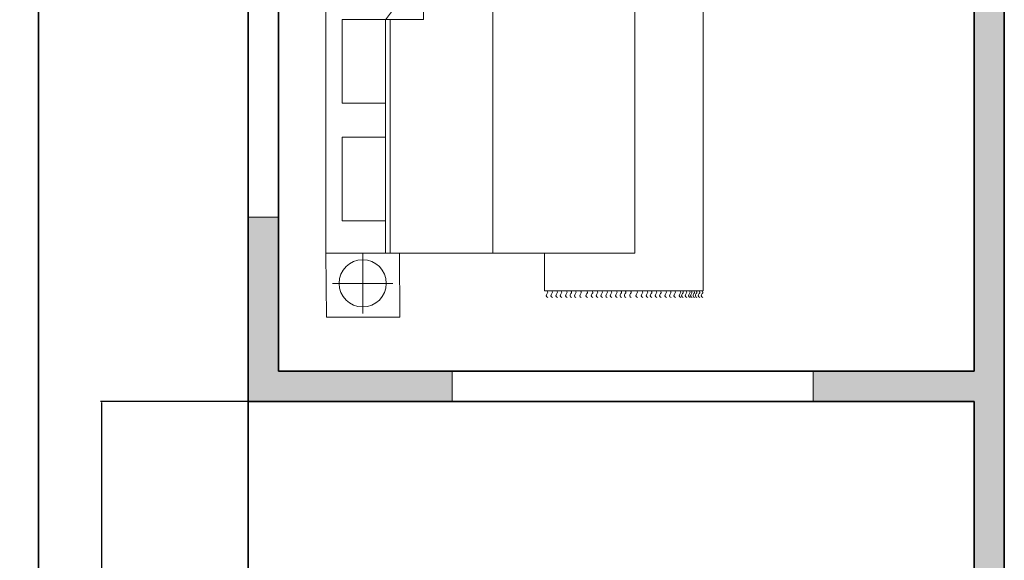
# Model space of a CAD drawing. Units: inches. Extents: x 717 to 1167, y 2046 to 2594.
# Tile 2 of 6: x 717 to 880, y 2208 to 2298. Entities that reach past the tile are written whole.
import ezdxf

# ---------------------------------------------------------------- set-up
doc = ezdxf.new("R2010")
doc.units = ezdxf.units.IN
doc.header["$MEASUREMENT"] = 0
for name, color, linetype, lineweight in [('A-ANNO-DIMS', 2, 'Continuous', 18), ('A-ANNO-TTLB', 7, 'Continuous', 35), ('A-FURN', 8, 'Continuous', 18), ('A-GLAZ', 4, 'Continuous', 18), ('A-WALL', 7, 'Continuous', 35), ('A-WALL-PATT', 140, 'Continuous', 13)]:
    doc.layers.add(name, color=color, linetype=linetype, lineweight=lineweight)
doc.styles.get("Standard").update_dxf_attribs({"font": 'arial.ttf'})
doc.dimstyles.get("Standard").update_dxf_attribs({"dimtxt": 6, "dimasz": 0.18, "dimexe": 0.18, "dimexo": 0.0625, "dimgap": 0.09, "dimtad": 0, "dimtih": 1, "dimtoh": 1, "dimdec": 1, "dimzin": 0, "dimdsep": 46, "dimlunit": 3, "dimtxsty": 'Standard', "dimcen": 0.09, "dimadec": 0, "dimazin": 0, "dimtfac": 1, "dimtdec": 1, "dimtofl": 0, "dimtmove": 0, "dimatfit": 3, "dimfxl": 1, "dimtolj": 1, "dimtzin": 0, "dimarcsym": 0})

# ---------------------------------------------------------------- blocks, each defined once
blk = doc.blocks.new('BED-DOUBLE-WITH-NIGHTSTANDS')
for p, q in [((6.09, 68.68), (6.09, 58.62)), ((36.42, 67.59), (62.78, 67.59)), ((36.42, 58.05), (36.42, 67.59)), ((62.78, 67.59), (62.78, 4.35)), ((1.07, 63.65), (11.12, 63.65)), ((9.97, 49.39), (16.32, 58)), ((16.32, 49.44), (16.32, 58)), ((27.82, 58.05), (27.82, 10.63)), ((9.97, 49.44), (16.32, 49.44)), ((9.97, 49.39), (9.97, 10.63)), ((10.78, 49.44), (10.78, 10.63)), ((6.2, 10.63), (6.2, 0.57)), ((36.42, 4.35), (36.42, 10.65)), ((1.17, 5.6), (11.22, 5.6)), ((62.78, 4.35), (36.42, 4.35))]:
    blk.add_line(p, q)
for points in [[(12.29, 58.05), (12.19, 68.68), (0, 68.68), (0.1, 58.05)], [(0.1, 58.05), (51.42, 58.05), (51.42, 10.63), (0.1, 10.63)], [(2.8, 49.44), (9.97, 49.44), (9.97, 35.55), (2.8, 35.55)], [(2.8, 29.88), (9.97, 29.88), (9.97, 15.98), (2.8, 15.98)], [(12.39, 0), (12.29, 10.63), (0.1, 10.63), (0.21, 0)]]:
    blk.add_lwpolyline(points, close=True)
for centre in [(6.09, 63.65), (6.2, 5.6)]:
    blk.add_circle(centre, 3.92)
for points, knots in [([(36.95, 68.71), (36.83, 68.61), (36.59, 68.42), (36.83, 68.08), (37, 67.8), (36.89, 67.65), (36.85, 67.58)], [0, 0, 0, 0, 0.400747, 0.791423, 1.067667, 1.29709, 1.29709, 1.29709, 1.29709]), ([(37.73, 68.71), (37.61, 68.61), (37.37, 68.42), (37.61, 68.08), (37.78, 67.8), (37.67, 67.65), (37.62, 67.58)], [0, 0, 0, 0, 0.400747, 0.791423, 1.067667, 1.29709, 1.29709, 1.29709, 1.29709]), ([(38.54, 68.71), (38.42, 68.61), (38.18, 68.42), (38.42, 68.08), (38.59, 67.8), (38.49, 67.65), (38.44, 67.58)], [0, 0, 0, 0, 0.400747, 0.791423, 1.067667, 1.29709, 1.29709, 1.29709, 1.29709]), ([(39.27, 68.71), (39.15, 68.61), (38.91, 68.42), (39.15, 68.08), (39.32, 67.8), (39.22, 67.65), (39.17, 67.58)], [0, 0, 0, 0, 0.400747, 0.791423, 1.067667, 1.29709, 1.29709, 1.29709, 1.29709]), ([(40.15, 68.71), (40.03, 68.61), (39.79, 68.42), (40.03, 68.08), (40.2, 67.8), (40.1, 67.65), (40.05, 67.58)], [0, 0, 0, 0, 0.400747, 0.791423, 1.067667, 1.29709, 1.29709, 1.29709, 1.29709]), ([(40.91, 68.71), (40.78, 68.61), (40.54, 68.42), (40.78, 68.08), (40.96, 67.8), (40.85, 67.65), (40.8, 67.58)], [0, 0, 0, 0, 0.400747, 0.791423, 1.067667, 1.29709, 1.29709, 1.29709, 1.29709]), ([(41.63, 68.71), (41.51, 68.61), (41.27, 68.42), (41.51, 68.08), (41.69, 67.8), (41.58, 67.65), (41.53, 67.58)], [0, 0, 0, 0, 0.400747, 0.791423, 1.067667, 1.29709, 1.29709, 1.29709, 1.29709]), ([(42.52, 68.71), (42.39, 68.61), (42.16, 68.42), (42.39, 68.08), (42.57, 67.8), (42.46, 67.65), (42.41, 67.58)], [0, 0, 0, 0, 0.400747, 0.791423, 1.067667, 1.29709, 1.29709, 1.29709, 1.29709]), ([(43.55, 68.71), (43.43, 68.61), (43.19, 68.42), (43.43, 68.08), (43.6, 67.8), (43.5, 67.65), (43.45, 67.58)], [0, 0, 0, 0, 0.400747, 0.791423, 1.067667, 1.29709, 1.29709, 1.29709, 1.29709]), ([(44.43, 68.71), (44.31, 68.61), (44.07, 68.42), (44.31, 68.08), (44.49, 67.8), (44.38, 67.65), (44.33, 67.58)], [0, 0, 0, 0, 0.400747, 0.791423, 1.067667, 1.29709, 1.29709, 1.29709, 1.29709]), ([(45.25, 68.71), (45.13, 68.61), (44.89, 68.42), (45.13, 68.08), (45.3, 67.8), (45.2, 67.65), (45.15, 67.58)], [0, 0, 0, 0, 0.400747, 0.791423, 1.067667, 1.29709, 1.29709, 1.29709, 1.29709]), ([(46.03, 68.71), (45.91, 68.61), (45.67, 68.42), (45.91, 68.08), (46.08, 67.8), (45.97, 67.65), (45.92, 67.58)], [0, 0, 0, 0, 0.400747, 0.791423, 1.067667, 1.29709, 1.29709, 1.29709, 1.29709]), ([(46.84, 68.71), (46.72, 68.61), (46.48, 68.42), (46.72, 68.08), (46.9, 67.8), (46.79, 67.65), (46.74, 67.58)], [0, 0, 0, 0, 0.400747, 0.791423, 1.067667, 1.29709, 1.29709, 1.29709, 1.29709]), ([(47.57, 68.71), (47.45, 68.61), (47.21, 68.42), (47.45, 68.08), (47.62, 67.8), (47.52, 67.65), (47.47, 67.58)], [0, 0, 0, 0, 0.400747, 0.791423, 1.067667, 1.29709, 1.29709, 1.29709, 1.29709]), ([(48.45, 68.71), (48.33, 68.61), (48.09, 68.42), (48.33, 68.08), (48.51, 67.8), (48.4, 67.65), (48.35, 67.58)], [0, 0, 0, 0, 0.400747, 0.791423, 1.067667, 1.29709, 1.29709, 1.29709, 1.29709]), ([(49.21, 68.71), (49.08, 68.61), (48.85, 68.42), (49.08, 68.08), (49.26, 67.8), (49.15, 67.65), (49.1, 67.58)], [0, 0, 0, 0, 0.400747, 0.791423, 1.067667, 1.29709, 1.29709, 1.29709, 1.29709]), ([(49.93, 68.71), (49.81, 68.61), (49.57, 68.42), (49.81, 68.08), (49.99, 67.8), (49.88, 67.65), (49.83, 67.58)], [0, 0, 0, 0, 0.400747, 0.791423, 1.067667, 1.29709, 1.29709, 1.29709, 1.29709]), ([(50.82, 68.71), (50.69, 68.61), (50.46, 68.42), (50.69, 68.08), (50.87, 67.8), (50.76, 67.65), (50.71, 67.58)], [0, 0, 0, 0, 0.400747, 0.791423, 1.067667, 1.29709, 1.29709, 1.29709, 1.29709]), ([(51.85, 68.71), (51.73, 68.61), (51.49, 68.42), (51.73, 68.08), (51.9, 67.8), (51.8, 67.65), (51.75, 67.58)], [0, 0, 0, 0, 0.400747, 0.791423, 1.067667, 1.29709, 1.29709, 1.29709, 1.29709]), ([(52.74, 68.71), (52.61, 68.61), (52.37, 68.42), (52.61, 68.08), (52.79, 67.8), (52.68, 67.65), (52.63, 67.58)], [0, 0, 0, 0, 0.400747, 0.791423, 1.067667, 1.29709, 1.29709, 1.29709, 1.29709]), ([(53.55, 68.71), (53.43, 68.61), (53.19, 68.42), (53.43, 68.08), (53.6, 67.8), (53.5, 67.65), (53.45, 67.58)], [0, 0, 0, 0, 0.400747, 0.791423, 1.067667, 1.29709, 1.29709, 1.29709, 1.29709]), ([(54.24, 68.71), (54.12, 68.61), (53.88, 68.42), (54.12, 68.08), (54.29, 67.8), (54.19, 67.65), (54.14, 67.58)], [0, 0, 0, 0, 0.400747, 0.791423, 1.067667, 1.29709, 1.29709, 1.29709, 1.29709]), ([(55.06, 68.71), (54.94, 68.61), (54.7, 68.42), (54.94, 68.08), (55.11, 67.8), (55, 67.65), (54.95, 67.58)], [0, 0, 0, 0, 0.400747, 0.791423, 1.067667, 1.29709, 1.29709, 1.29709, 1.29709]), ([(55.78, 68.71), (55.66, 68.61), (55.42, 68.42), (55.66, 68.08), (55.84, 67.8), (55.73, 67.65), (55.68, 67.58)], [0, 0, 0, 0, 0.400747, 0.791423, 1.067667, 1.29709, 1.29709, 1.29709, 1.29709]), ([(56.67, 68.71), (56.55, 68.61), (56.31, 68.42), (56.55, 68.08), (56.72, 67.8), (56.61, 67.65), (56.56, 67.58)], [0, 0, 0, 0, 0.400747, 0.791423, 1.067667, 1.29709, 1.29709, 1.29709, 1.29709]), ([(57.42, 68.71), (57.3, 68.61), (57.06, 68.42), (57.3, 68.08), (57.47, 67.8), (57.36, 67.65), (57.32, 67.58)], [0, 0, 0, 0, 0.400747, 0.791423, 1.067667, 1.29709, 1.29709, 1.29709, 1.29709]), ([(58.15, 68.71), (58.03, 68.61), (57.79, 68.42), (58.03, 68.08), (58.2, 67.8), (58.1, 67.66), (58.05, 67.59)], [0, 0, 0, 0, 0.400747, 0.791423, 1.067667, 1.283686, 1.283686, 1.283686, 1.283686]), ([(59.03, 68.71), (58.91, 68.61), (58.67, 68.42), (58.91, 68.08), (59.08, 67.8), (58.98, 67.66), (58.93, 67.59)], [0, 0, 0, 0, 0.400747, 0.791423, 1.067667, 1.283686, 1.283686, 1.283686, 1.283686]), ([(59.46, 68.71), (59.34, 68.61), (59.09, 68.42), (59.34, 68.08), (59.51, 67.8), (59.41, 67.66), (59.36, 67.59)], [0, 0, 0, 0, 0.402903, 0.794912, 1.071156, 1.287177, 1.287177, 1.287177, 1.287177]), ([(60.05, 68.71), (59.93, 68.61), (59.69, 68.42), (59.93, 68.08), (60.1, 67.8), (60, 67.66), (59.96, 67.59)], [0, 0, 0, 0, 0.400747, 0.791423, 1.067667, 1.283686, 1.283686, 1.283686, 1.283686]), ([(60.63, 68.71), (60.51, 68.61), (60.27, 68.42), (60.51, 68.08), (60.68, 67.8), (60.58, 67.66), (60.53, 67.59)], [0, 0, 0, 0, 0.400747, 0.791423, 1.067667, 1.283686, 1.283686, 1.283686, 1.283686]), ([(60.94, 68.71), (60.82, 68.61), (60.58, 68.42), (60.81, 68.08), (60.99, 67.8), (60.89, 67.66), (60.84, 67.59)], [0, 0, 0, 0, 0.400747, 0.791423, 1.067667, 1.283686, 1.283686, 1.283686, 1.283686]), ([(61.36, 68.71), (61.23, 68.61), (60.99, 68.42), (61.23, 68.08), (61.41, 67.8), (61.3, 67.65), (61.25, 67.58)], [0, 0, 0, 0, 0.400747, 0.791423, 1.067667, 1.29709, 1.29709, 1.29709, 1.29709]), ([(61.75, 68.71), (61.63, 68.61), (61.39, 68.42), (61.63, 68.08), (61.8, 67.8), (61.7, 67.65), (61.65, 67.58)], [0, 0, 0, 0, 0.400747, 0.791423, 1.067667, 1.29709, 1.29709, 1.29709, 1.29709]), ([(62.24, 68.71), (62.12, 68.61), (61.88, 68.42), (62.12, 68.08), (62.29, 67.8), (62.18, 67.65), (62.13, 67.58)], [0, 0, 0, 0, 0.400747, 0.791423, 1.067667, 1.29709, 1.29709, 1.29709, 1.29709]), ([(62.71, 68.71), (62.59, 68.61), (62.35, 68.42), (62.59, 68.08), (62.76, 67.8), (62.66, 67.65), (62.61, 67.58)], [0, 0, 0, 0, 0.400747, 0.791423, 1.067667, 1.29709, 1.29709, 1.29709, 1.29709]), ([(36.95, 3.23), (36.83, 3.32), (36.59, 3.52), (36.83, 3.86), (37, 4.14), (36.89, 4.29), (36.85, 4.35)], [0, 0, 0, 0, 0.400747, 0.791423, 1.067667, 1.29709, 1.29709, 1.29709, 1.29709]), ([(37.73, 3.23), (37.61, 3.32), (37.37, 3.52), (37.61, 3.86), (37.78, 4.14), (37.67, 4.29), (37.62, 4.35)], [0, 0, 0, 0, 0.400747, 0.791423, 1.067667, 1.29709, 1.29709, 1.29709, 1.29709]), ([(38.54, 3.23), (38.42, 3.32), (38.18, 3.52), (38.42, 3.86), (38.59, 4.14), (38.49, 4.29), (38.44, 4.35)], [0, 0, 0, 0, 0.400747, 0.791423, 1.067667, 1.29709, 1.29709, 1.29709, 1.29709]), ([(39.27, 3.23), (39.15, 3.32), (38.91, 3.52), (39.15, 3.86), (39.32, 4.14), (39.22, 4.29), (39.17, 4.35)], [0, 0, 0, 0, 0.400747, 0.791423, 1.067667, 1.29709, 1.29709, 1.29709, 1.29709]), ([(40.15, 3.23), (40.03, 3.32), (39.79, 3.52), (40.03, 3.86), (40.2, 4.14), (40.1, 4.29), (40.05, 4.35)], [0, 0, 0, 0, 0.400747, 0.791423, 1.067667, 1.29709, 1.29709, 1.29709, 1.29709]), ([(40.91, 3.23), (40.78, 3.32), (40.54, 3.52), (40.78, 3.86), (40.96, 4.14), (40.85, 4.29), (40.8, 4.35)], [0, 0, 0, 0, 0.400747, 0.791423, 1.067667, 1.29709, 1.29709, 1.29709, 1.29709]), ([(41.63, 3.23), (41.51, 3.32), (41.27, 3.52), (41.51, 3.86), (41.69, 4.14), (41.58, 4.29), (41.53, 4.35)], [0, 0, 0, 0, 0.400747, 0.791423, 1.067667, 1.29709, 1.29709, 1.29709, 1.29709]), ([(42.52, 3.23), (42.39, 3.32), (42.16, 3.52), (42.39, 3.86), (42.57, 4.14), (42.46, 4.29), (42.41, 4.35)], [0, 0, 0, 0, 0.400747, 0.791423, 1.067667, 1.29709, 1.29709, 1.29709, 1.29709]), ([(43.55, 3.23), (43.43, 3.32), (43.19, 3.52), (43.43, 3.86), (43.6, 4.14), (43.5, 4.29), (43.45, 4.35)], [0, 0, 0, 0, 0.400747, 0.791423, 1.067667, 1.29709, 1.29709, 1.29709, 1.29709]), ([(44.43, 3.23), (44.31, 3.32), (44.07, 3.52), (44.31, 3.86), (44.49, 4.14), (44.38, 4.29), (44.33, 4.35)], [0, 0, 0, 0, 0.400747, 0.791423, 1.067667, 1.29709, 1.29709, 1.29709, 1.29709]), ([(45.25, 3.23), (45.13, 3.32), (44.89, 3.52), (45.13, 3.86), (45.3, 4.14), (45.2, 4.29), (45.15, 4.35)], [0, 0, 0, 0, 0.400747, 0.791423, 1.067667, 1.29709, 1.29709, 1.29709, 1.29709]), ([(46.03, 3.23), (45.91, 3.32), (45.67, 3.52), (45.91, 3.86), (46.08, 4.14), (45.97, 4.29), (45.92, 4.35)], [0, 0, 0, 0, 0.400747, 0.791423, 1.067667, 1.29709, 1.29709, 1.29709, 1.29709]), ([(46.84, 3.23), (46.72, 3.32), (46.48, 3.52), (46.72, 3.86), (46.9, 4.14), (46.79, 4.29), (46.74, 4.35)], [0, 0, 0, 0, 0.400747, 0.791423, 1.067667, 1.29709, 1.29709, 1.29709, 1.29709]), ([(47.57, 3.23), (47.45, 3.32), (47.21, 3.52), (47.45, 3.86), (47.62, 4.14), (47.52, 4.29), (47.47, 4.35)], [0, 0, 0, 0, 0.400747, 0.791423, 1.067667, 1.29709, 1.29709, 1.29709, 1.29709]), ([(48.45, 3.23), (48.33, 3.32), (48.09, 3.52), (48.33, 3.86), (48.51, 4.14), (48.4, 4.29), (48.35, 4.35)], [0, 0, 0, 0, 0.400747, 0.791423, 1.067667, 1.29709, 1.29709, 1.29709, 1.29709]), ([(49.21, 3.23), (49.08, 3.32), (48.85, 3.52), (49.08, 3.86), (49.26, 4.14), (49.15, 4.29), (49.1, 4.35)], [0, 0, 0, 0, 0.400747, 0.791423, 1.067667, 1.29709, 1.29709, 1.29709, 1.29709]), ([(49.93, 3.23), (49.81, 3.32), (49.57, 3.52), (49.81, 3.86), (49.99, 4.14), (49.88, 4.29), (49.83, 4.35)], [0, 0, 0, 0, 0.400747, 0.791423, 1.067667, 1.29709, 1.29709, 1.29709, 1.29709]), ([(50.82, 3.23), (50.69, 3.32), (50.46, 3.52), (50.69, 3.86), (50.87, 4.14), (50.76, 4.29), (50.71, 4.35)], [0, 0, 0, 0, 0.400747, 0.791423, 1.067667, 1.29709, 1.29709, 1.29709, 1.29709]), ([(51.85, 3.23), (51.73, 3.32), (51.49, 3.52), (51.73, 3.86), (51.9, 4.14), (51.8, 4.29), (51.75, 4.35)], [0, 0, 0, 0, 0.400747, 0.791423, 1.067667, 1.29709, 1.29709, 1.29709, 1.29709]), ([(52.74, 3.23), (52.61, 3.32), (52.37, 3.52), (52.61, 3.86), (52.79, 4.14), (52.68, 4.29), (52.63, 4.35)], [0, 0, 0, 0, 0.400747, 0.791423, 1.067667, 1.29709, 1.29709, 1.29709, 1.29709]), ([(53.55, 3.23), (53.43, 3.32), (53.19, 3.52), (53.43, 3.86), (53.6, 4.14), (53.5, 4.29), (53.45, 4.35)], [0, 0, 0, 0, 0.400747, 0.791423, 1.067667, 1.29709, 1.29709, 1.29709, 1.29709]), ([(54.24, 3.23), (54.12, 3.32), (53.88, 3.52), (54.12, 3.86), (54.29, 4.14), (54.19, 4.29), (54.14, 4.35)], [0, 0, 0, 0, 0.400747, 0.791423, 1.067667, 1.29709, 1.29709, 1.29709, 1.29709]), ([(55.06, 3.23), (54.94, 3.32), (54.7, 3.52), (54.94, 3.86), (55.11, 4.14), (55, 4.29), (54.95, 4.35)], [0, 0, 0, 0, 0.400747, 0.791423, 1.067667, 1.29709, 1.29709, 1.29709, 1.29709]), ([(55.78, 3.23), (55.66, 3.32), (55.42, 3.52), (55.66, 3.86), (55.84, 4.14), (55.73, 4.29), (55.68, 4.35)], [0, 0, 0, 0, 0.400747, 0.791423, 1.067667, 1.29709, 1.29709, 1.29709, 1.29709]), ([(56.67, 3.23), (56.55, 3.32), (56.31, 3.52), (56.55, 3.86), (56.72, 4.14), (56.61, 4.29), (56.56, 4.35)], [0, 0, 0, 0, 0.400747, 0.791423, 1.067667, 1.29709, 1.29709, 1.29709, 1.29709]), ([(57.42, 3.23), (57.3, 3.32), (57.06, 3.52), (57.3, 3.86), (57.47, 4.14), (57.36, 4.29), (57.32, 4.35)], [0, 0, 0, 0, 0.400747, 0.791423, 1.067667, 1.29709, 1.29709, 1.29709, 1.29709]), ([(58.15, 3.23), (58.03, 3.32), (57.79, 3.52), (58.03, 3.86), (58.2, 4.14), (58.09, 4.29), (58.04, 4.35)], [0, 0, 0, 0, 0.400747, 0.791423, 1.067667, 1.29709, 1.29709, 1.29709, 1.29709]), ([(59.03, 3.23), (58.91, 3.32), (58.67, 3.52), (58.91, 3.86), (59.08, 4.14), (58.98, 4.29), (58.93, 4.35)], [0, 0, 0, 0, 0.400747, 0.791423, 1.067667, 1.29709, 1.29709, 1.29709, 1.29709]), ([(59.46, 3.23), (59.33, 3.32), (59.08, 3.51), (59.34, 3.86), (59.51, 4.14), (59.4, 4.29), (59.36, 4.35)], [0, 0, 0, 0, 0.407265, 0.802015, 1.07826, 1.307683, 1.307683, 1.307683, 1.307683]), ([(60.03, 3.23), (59.9, 3.32), (59.67, 3.52), (59.9, 3.86), (60.08, 4.14), (59.97, 4.29), (59.92, 4.35)], [0, 0, 0, 0, 0.400747, 0.791423, 1.067667, 1.29709, 1.29709, 1.29709, 1.29709]), ([(60.6, 3.23), (60.48, 3.32), (60.24, 3.52), (60.48, 3.86), (60.65, 4.14), (60.54, 4.29), (60.5, 4.35)], [0, 0, 0, 0, 0.400747, 0.791423, 1.067667, 1.29709, 1.29709, 1.29709, 1.29709]), ([(60.91, 3.23), (60.79, 3.32), (60.55, 3.52), (60.79, 3.86), (60.96, 4.14), (60.85, 4.29), (60.81, 4.35)], [0, 0, 0, 0, 0.400747, 0.791423, 1.067667, 1.29709, 1.29709, 1.29709, 1.29709]), ([(61.33, 3.23), (61.21, 3.32), (60.97, 3.52), (61.21, 3.86), (61.38, 4.14), (61.27, 4.29), (61.22, 4.35)], [0, 0, 0, 0, 0.400747, 0.791423, 1.067667, 1.29709, 1.29709, 1.29709, 1.29709]), ([(61.72, 3.23), (61.6, 3.32), (61.36, 3.52), (61.6, 3.86), (61.78, 4.14), (61.67, 4.29), (61.62, 4.35)], [0, 0, 0, 0, 0.400747, 0.791423, 1.067667, 1.29709, 1.29709, 1.29709, 1.29709]), ([(62.21, 3.23), (62.09, 3.32), (61.85, 3.52), (62.09, 3.86), (62.26, 4.14), (62.15, 4.29), (62.11, 4.35)], [0, 0, 0, 0, 0.400747, 0.791423, 1.067667, 1.29709, 1.29709, 1.29709, 1.29709]), ([(62.71, 3.23), (62.59, 3.32), (62.35, 3.52), (62.59, 3.86), (62.76, 4.14), (62.66, 4.29), (62.61, 4.35)], [0, 0, 0, 0, 0.400747, 0.791423, 1.067667, 1.29709, 1.29709, 1.29709, 1.29709])]:
    blk.add_open_spline(points, degree=3, knots=knots)
blk = doc.blocks.new('WINDOW-60IN')
for p, q in [((0, 5), (0, 0)), ((60, 5), (0, 5)), ((60, 0), (60, 5)), ((0, 0), (60, 0))]:
    blk.add_line(p, q)
blk = doc.blocks.new('*D34')
at = {"layer": 'A-ANNO-DIMS', "color": 0, "lineweight": -2, "transparency": 16777216}
for p, q in [((754.65, 2234.77), (730.13, 2234.77)), ((730.31, 2234.59), (730.31, 2160.27)), ((730.31, 2079.75), (730.31, 2154.07)), ((754.65, 2079.57), (730.13, 2079.57))]:
    blk.add_line(p, q, dxfattribs=at)
at = {"layer": 'A-ANNO-DIMS', "color": 0, "transparency": 16777216}
for points in [[(730.28, 2234.59), (730.34, 2234.59), (730.31, 2234.77)], [(730.28, 2079.75), (730.34, 2079.75), (730.31, 2079.57)]]:
    blk.add_solid(points, dxfattribs=at)
at = {"layer": 'Defpoints', "color": 0, "transparency": 16777216}
for p in [(730.31, 2234.77), (754.71, 2234.77), (754.71, 2079.57)]:
    blk.add_point(p, dxfattribs=at)
at = {"layer": 'A-ANNO-DIMS', "color": 0, "transparency": 16777216, "insert": (730.31, 2157.17), "char_height": 6, "attachment_point": 5}
blk.add_mtext('\\A1;12\'-11"', dxfattribs=at)

msp = doc.modelspace()

# ---------------------------------------------------------------- hatches: boundary and pattern name
at = {"layer": 'A-WALL-PATT'}
h = msp.add_hatch(color=256, dxfattribs=at)
h.dxf.hatch_style = 1
h.paths.add_polyline_path([(796.2, 2547.57), (754.71, 2547.57), (754.71, 2325.38), (759.71, 2325.38), (759.71, 2357.37), (840.31, 2357.37), (840.31, 2362.37), (759.71, 2362.37), (759.71, 2412.77), (835.31, 2412.77), (835.31, 2386.37), (840.31, 2386.37), (840.31, 2412.77), (901.51, 2412.77), (901.51, 2417.77), (759.71, 2417.77), (759.71, 2542.57), (796.2, 2542.57)])
h.paths.add_polyline_path([(913.34, 2547.57), (856.2, 2547.57), (856.2, 2542.57), (896.51, 2542.57), (896.51, 2453.77), (901.51, 2453.77), (901.51, 2542.57), (913.34, 2542.57)])
h.paths.add_polyline_path([(1012.57, 2547.57), (949.34, 2547.57), (949.34, 2542.57), (967.91, 2542.57), (967.91, 2412.77), (972.91, 2412.77), (972.91, 2542.57), (1012.57, 2542.57)])
h.paths.add_polyline_path([(1114.71, 2547.57), (1072.57, 2547.57), (1072.57, 2542.57), (1109.71, 2542.57), (1109.71, 2517.4), (1114.71, 2517.4)])
h.paths.add_polyline_path([(1114.71, 2457.4), (1109.71, 2457.4), (1109.71, 2393.68), (1114.71, 2393.68)])
h.paths.add_polyline_path([(1114.71, 2369.68), (1109.71, 2369.68), (1109.71, 2362.37), (1038.91, 2362.37), (1038.91, 2412.77), (1085.71, 2412.77), (1085.71, 2417.77), (1008.91, 2417.77), (1008.91, 2412.77), (1033.91, 2412.77), (1033.91, 2362.37), (916.31, 2362.37), (916.31, 2357.37), (1033.91, 2357.37), (1033.91, 2306.97), (1003.91, 2306.97), (1003.91, 2301.97), (1085.71, 2301.97), (1085.71, 2306.97), (1038.91, 2306.97), (1038.91, 2357.37), (1109.71, 2357.37), (1109.71, 2347.44), (1114.71, 2347.44)])
h.paths.add_polyline_path([(788.58, 2239.77), (759.71, 2239.77), (759.71, 2265.38), (754.71, 2265.38), (754.71, 2234.77), (788.58, 2234.77)])
h.paths.add_polyline_path([(880.31, 2362.37), (875.31, 2362.37), (875.31, 2239.77), (848.58, 2239.77), (848.58, 2234.77), (875.31, 2234.77), (875.31, 2079.57), (880.31, 2079.57)])
h.paths.add_polyline_path([(1008.91, 2265.97), (1003.91, 2265.97), (1003.91, 2127.77), (991.51, 2127.77), (991.51, 2122.77), (1003.91, 2122.77), (1003.91, 2079.57), (1036.96, 2079.57), (1036.96, 2084.57), (1008.91, 2084.57)])
h.paths.add_polyline_path([(931.51, 2127.77), (916.31, 2127.77), (916.31, 2122.77), (931.51, 2122.77)])
h.paths.add_polyline_path([(1114.71, 2162.57), (1109.71, 2162.57), (1109.71, 2084.57), (1096.96, 2084.57), (1096.96, 2079.57), (1114.71, 2079.57)])
h.paths.add_polyline_path([(1114.71, 2211.37), (1109.71, 2211.37), (1109.71, 2191.57), (1044.91, 2191.57), (1044.91, 2186.57), (1114.71, 2186.57)])
h.paths.add_polyline_path([(1114.71, 2323.44), (1109.71, 2323.44), (1109.71, 2271.37), (1114.71, 2271.37)])

# ---------------------------------------------------------------- linework, layer by layer
at = {"layer": 'A-ANNO-TTLB'}
msp.add_lwpolyline([(719.86, 2594.22), (1167.21, 2594.22), (1167.21, 2050.08), (719.86, 2050.08)], close=True, dxfattribs=at)
at = {"layer": 'A-WALL'}
for p, q in [((754.71, 2547.57), (754.71, 2079.57)), ((875.31, 2362.37), (875.31, 2239.77)), ((880.31, 2362.37), (880.31, 2079.57)), ((759.71, 2357.37), (759.71, 2239.77)), ((759.71, 2239.77), (875.31, 2239.77)), ((754.71, 2234.77), (875.31, 2234.77)), ((875.31, 2234.77), (875.31, 2079.57))]:
    msp.add_line(p, q, dxfattribs=at)

# ---------------------------------------------------------------- block references
at = {"layer": 'A-FURN'}
msp.add_blockref('BED-DOUBLE-WITH-NIGHTSTANDS', (767.52, 2248.78), dxfattribs=at)
at = {"layer": 'A-GLAZ', "rotation": 270}
msp.add_blockref('WINDOW-60IN', (754.71, 2325.38), dxfattribs=at)
at = {"layer": 'A-GLAZ'}
msp.add_blockref('WINDOW-60IN', (788.58, 2234.77), dxfattribs=at)

# ---------------------------------------------------------------- dimensions: what is measured, and where the dimension line sits
at = {"layer": 'A-ANNO-DIMS'}
dim = msp.add_linear_dim(base=(730.31, 2234.77), p1=(754.71, 2079.57), p2=(754.71, 2234.77), angle=90, dimstyle='Standard', override={"dimdec": 1, "dimlfac": 1, "dimrnd": 0, "dimzin": 1, "dimdsep": 46, "dimlunit": 4, "dimfrac": 2}, dxfattribs=at)
dim.commit()
dim.dimension.update_dxf_attribs({"geometry": '*D34', "text_midpoint": (730.31, 2157.17)})

doc.saveas('drawing.dxf')
